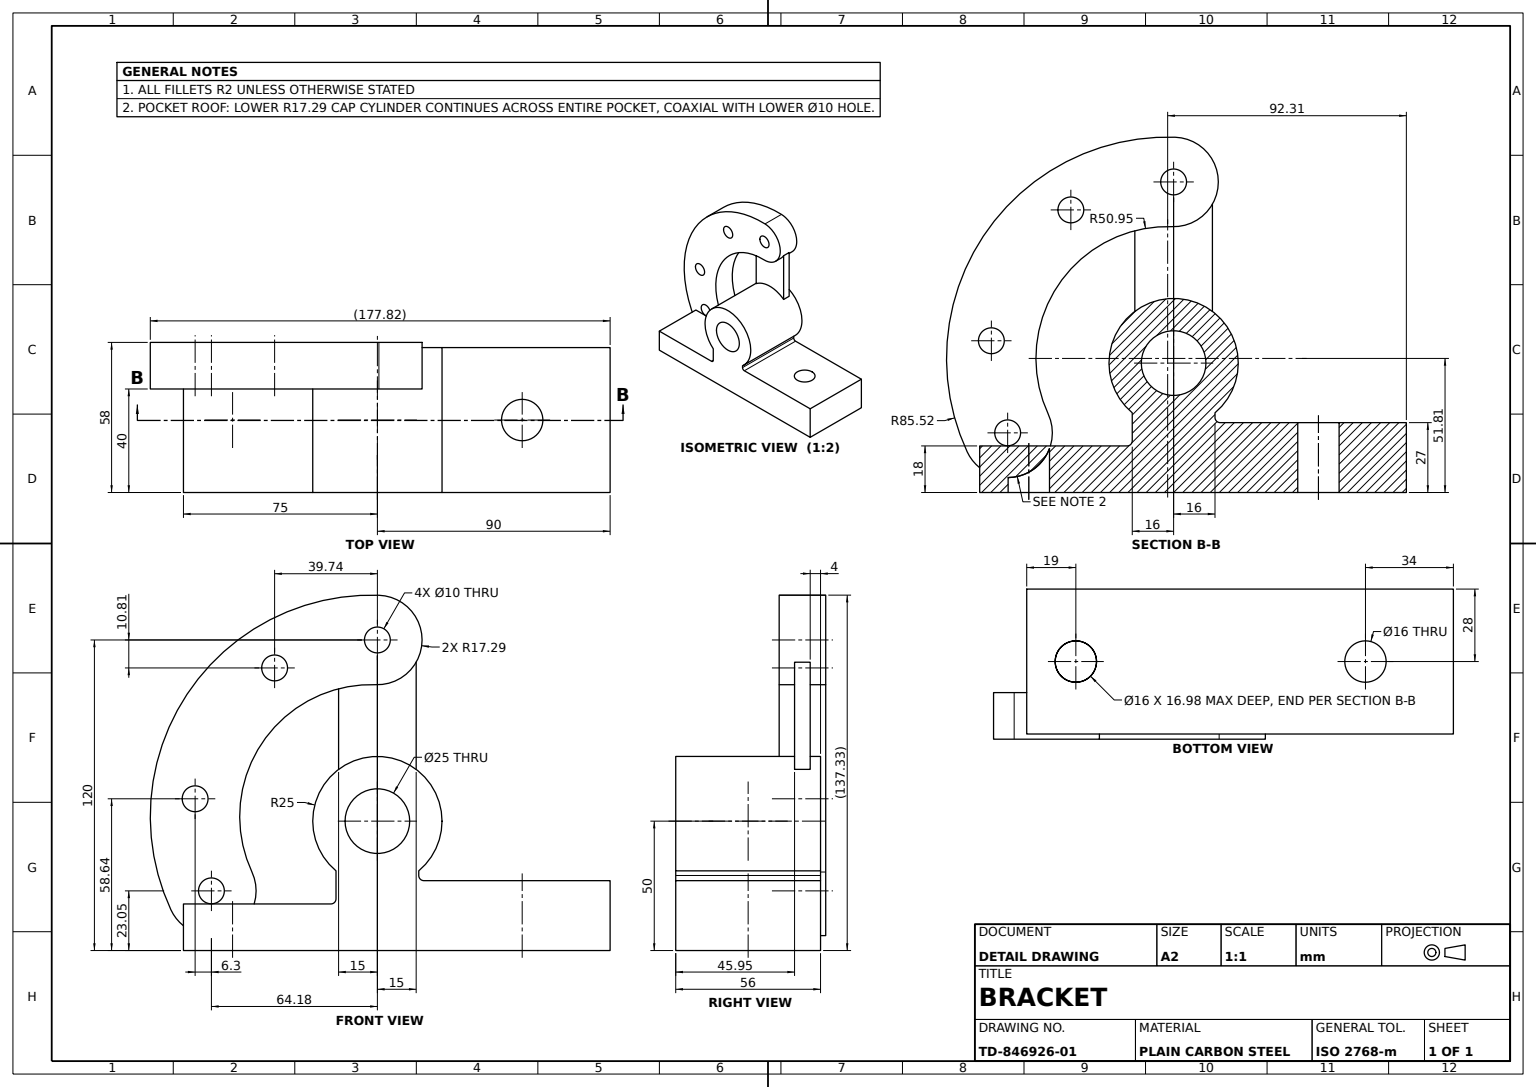
from build123d import *

# Parameters (mm, degrees)
BASE_PLATE_DEPTH            = 56
HUB_BOSS_SKETCH_R           = 12.5
HUB_BOSS_DEPTH              = 56
HUB_FILLET_R2_R             = 2
WEB_SKETCH_W                = 30
WEB_SKETCH_H                = 54.40435867
WEB_4MM_DEPTH               = 52
HUB_BORE_REACH              = 162.112
HUB_BORE_END_RADIUS         = 25
HUB_BORE_SKETCH_W           = 30
HUB_BORE_SKETCH_H           = 45.952641166
FLANGE_PLATE_DEPTH          = 58
FLANGE_SLOT_CUT_DEPTH       = 40
FLANGE_BOLT_HOLES_SKETCH_R  = 5
FLANGE_BOLT_HOLES_DEPTH     = 40
BASE_MOUNTING_HOLE_SKETCH_R = 8
BASE_MOUNTING_HOLE_DEPTH    = 154.738826956
FLANGE_CLOSING_BOSS_DEPTH   = 40


with BuildPart() as part:
    # Base Plate Sketch → Base Plate (new body)
    with BuildSketch(Plane.XY):
        Polygon((0, 0), (-75, 0), (-75, 18), (0, 18), (0, 27), (90, 27), (90, 0), align=None)
    extrude(amount=-BASE_PLATE_DEPTH)

    # Hub Boss Sketch → Hub Boss (add)
    with BuildSketch(Plane.XY):
        with BuildLine():
            Line((-16, 30.790627288), (-16, 18))
            Line((-16, 18), (16, 18))
            Line((16, 18), (16, 30.790627288))
            ThreePointArc((16, 30.790627288), (0, 75), (-16, 30.790627288))
        make_face()
        with Locations((0, 50)):
            Circle(HUB_BOSS_SKETCH_R, mode=Mode.SUBTRACT)
    extrude(amount=-HUB_BOSS_DEPTH)

    # Hub Fillet R2
    hub_fillet_r2_edges = [part.edges().sort_by_distance(p)[0] for p in [
        (16, 27, -28),
        (-16, 18, -28),
    ]]
    fillet(hub_fillet_r2_edges, radius=HUB_FILLET_R2_R)

    # Web Sketch → Web 4mm (add)
    with BuildSketch(Plane.XY):
        with Locations((0, 92.797820665)):
            Rectangle(WEB_SKETCH_W, WEB_SKETCH_H)
    extrude(amount=-WEB_4MM_DEPTH)

    # Hub Bore: up to this cylinder (the profile starts outside it)
    hub_bore_end = Plane(origin=(0, 50, -22.976321), z_dir=(0, 0, 1)) * Cylinder(HUB_BORE_END_RADIUS, 375.224, mode=Mode.PRIVATE)
    # Hub Bore Sketch → Hub Bore (cut, up to the surface)
    with BuildSketch(Plane(origin=(0, 120, 0), x_dir=(1, 0, 0), z_dir=(0, 1, 0)), mode=Mode.PRIVATE) as hub_bore_sk1:
        with Locations((0, 22.976320583)):
            Rectangle(HUB_BORE_SKETCH_W, HUB_BORE_SKETCH_H)
    hub_bore_tool1 = extrude(hub_bore_sk1.sketch, amount=-HUB_BORE_REACH, mode=Mode.PRIVATE) - hub_bore_end
    add(hub_bore_tool1.solids().sort_by_distance((0, 120, -22.976321))[0], mode=Mode.SUBTRACT)

    # Flange Profile Sketch → Flange Plate (add)
    with BuildSketch(Plane.XY):
        with BuildLine():
            ThreePointArc((0.584249397, 137.276236883), (-73.612691272, 99.015664074), (-79.858671486, 15.768771234))
            ThreePointArc((-79.858671486, 15.768771234), (-56.897741093, 7.377401147), (-48.506371007, 30.33833154))
            ThreePointArc((-48.506371007, 30.33833154), (-44.785464057, 79.930858496), (-0.584249397, 102.723763117))
            ThreePointArc((-0.584249397, 102.723763117), (17.276236883, 119.415750603), (0.584249397, 137.276236883))
        make_face()
    extrude(amount=-FLANGE_PLATE_DEPTH)

    # Sketch7_2 → Flange Slot Cut (cut)
    with BuildSketch(Plane.XY):
        with BuildLine():
            ThreePointArc((0.584249397, 137.276236883), (-73.612691272, 99.015664074), (-79.858671486, 15.768771234))
            ThreePointArc((-79.858671486, 15.768771234), (-56.897741093, 7.377401147), (-48.506371007, 30.33833154))
            ThreePointArc((-48.506371007, 30.33833154), (-44.785464057, 79.930858496), (-0.584249397, 102.723763117))
            ThreePointArc((-0.584249397, 102.723763117), (17.276236883, 119.415750603), (0.584249397, 137.276236883))
        make_face()
    extrude(amount=-FLANGE_SLOT_CUT_DEPTH, mode=Mode.SUBTRACT)

    # Flange Bolt Holes Sketch → Flange Bolt Holes (cut)
    with BuildSketch(Plane(origin=(0, 0, -58), x_dir=(-1, 0, 0), z_dir=(0, 0, -1))):
        with Locations((0, 120)):
            Circle(FLANGE_BOLT_HOLES_SKETCH_R)
        with Locations((39.743102788, 109.193277489)):
            Circle(FLANGE_BOLT_HOLES_SKETCH_R)
        with Locations((70.482390924, 58.635502651)):
            Circle(FLANGE_BOLT_HOLES_SKETCH_R)
        with Locations((64.182521246, 23.053551387)):
            Circle(FLANGE_BOLT_HOLES_SKETCH_R)
    extrude(amount=-FLANGE_BOLT_HOLES_DEPTH, mode=Mode.SUBTRACT)

    # Base Mounting Hole Sketch → Base Mounting Hole (cut, through all)
    with BuildSketch(Plane(origin=(0, 27, 0), x_dir=(1, 0, 0), z_dir=(0, 1, 0))):
        with Locations(Location((56, 28, 0), (0, 0, 270))):
            Circle(BASE_MOUNTING_HOLE_SKETCH_R)
        with Locations(Location((-56, 28, 0), (0, 0, 270))):
            Circle(BASE_MOUNTING_HOLE_SKETCH_R)
    extrude(amount=-BASE_MOUNTING_HOLE_DEPTH, mode=Mode.SUBTRACT)

    # Flange Closing Boss Sketch → Flange Closing Boss (add)
    with BuildSketch(Plane.XY):
        with BuildLine():
            Line((-47.651600927, 18), (-75, 18))
            Line((-75, 18), (-75, 9.570530152))
            ThreePointArc((-75, 9.570530152), (-59.090876707, 6.534324283), (-47.651600927, 18))
        make_face()
    extrude(amount=-FLANGE_CLOSING_BOSS_DEPTH)


solid = part.part
